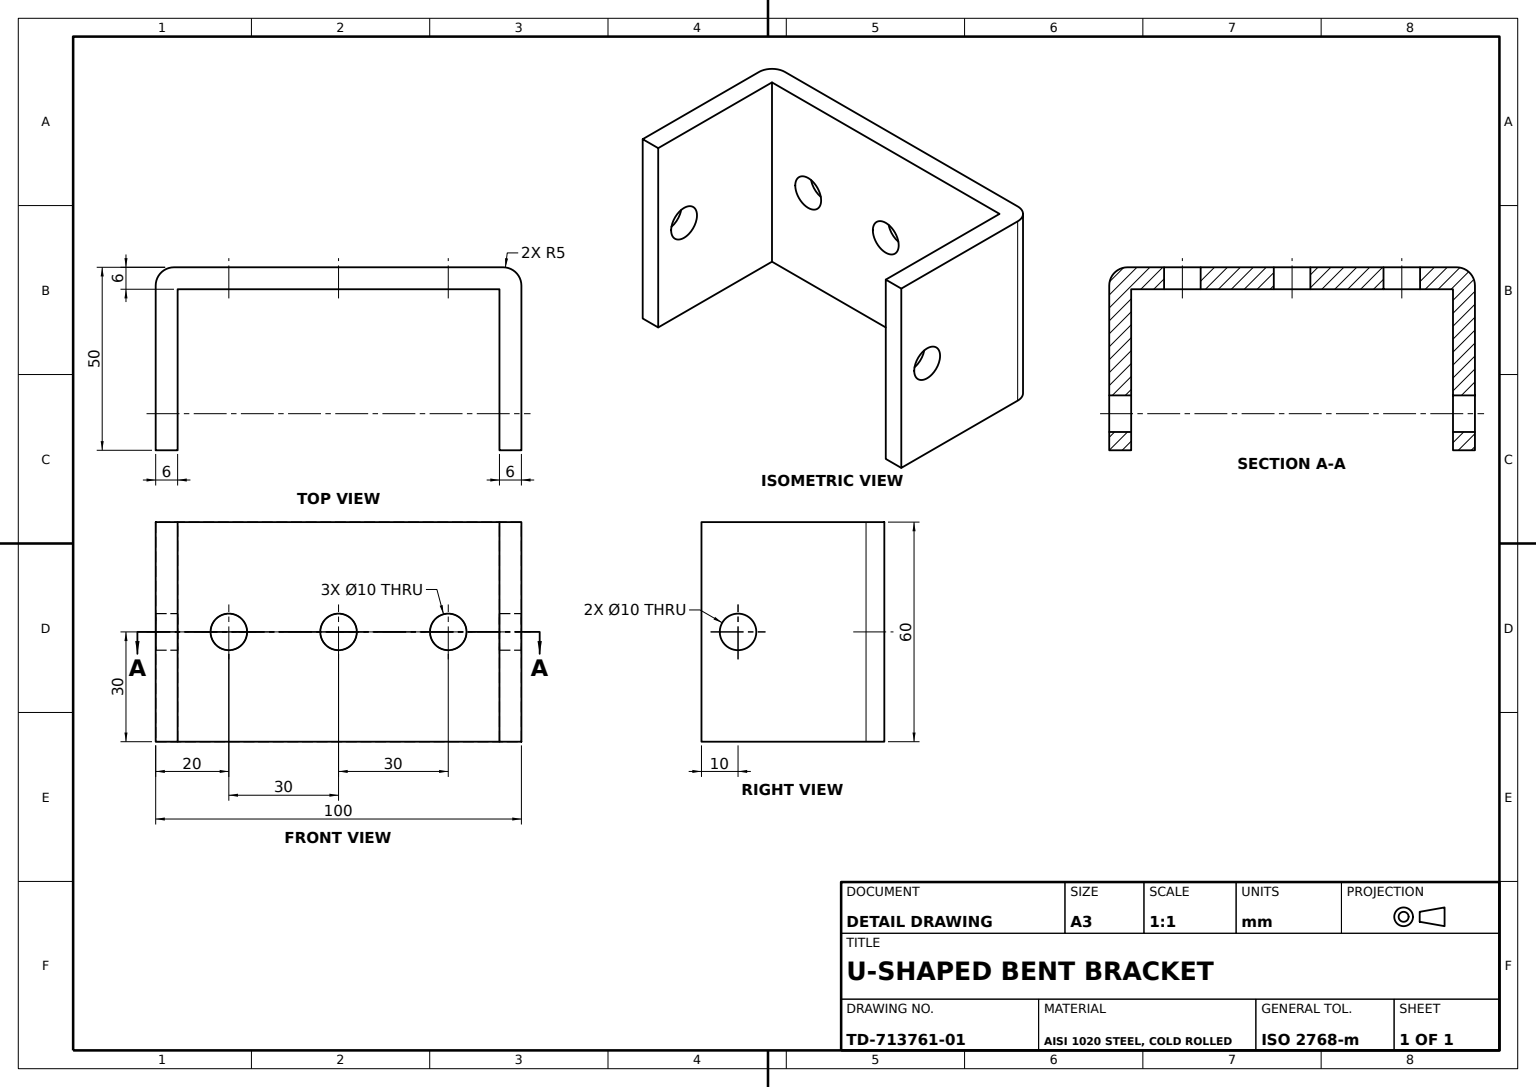
SolidWorks part; units mm, degrees
material "AISI 1020 Steel, Cold Rolled"
ref_plane "Front Plane" through (0, 0, 0) normal (0, 0, 1) x (1, 0, 0)
ref_plane "Top Plane" through (0, 0, 0) normal (0, 1, 0) x (1, 0, 0)
ref_plane "Right Plane" through (0, 0, 0) normal (1, 0, 0) x (0, 0, -1)
sketch "Channel Profile Sketch" plane through (0, 0, 0) normal (0, 1, 0) x (1, 0, 0)
  line L0 (0, 0) -> (0, 50)
  line L1 (0, 50) -> (100, 50)
  line L2 (100, 50) -> (100, 0)
  line L4 (100, 0) -> (94, 0)
  line L5 (94, 0) -> (94, 44)
  line L6 (94, 44) -> (6, 44)
  line L7 (6, 44) -> (6, 0)
  line L8 (6, 0) -> (0, 0)
  dimension "D1" = 50
  dimension "D2" = 100
  dimension "D3" = 6
  dimension "D4" = 6
  dimension "D5" = 6
extrude "Channel Body" add sketch "Channel Profile Sketch" against normal mid plane 60
sketch "Flange Holes Sketch" plane through (0, 0, -50) normal (0, 0, -1) x (-1, 0, 0)
  line L0 (0, 0) -> (-343.6549, 0) construction
  line L1 (-50, -30) -> (-50, 63.2025) construction
  line L2 (-100, -30) -> (0, -30) construction
  circle A0 centre (-50, 0) radius 5
  circle A1 centre (-20, 0) radius 5
  circle A2 centre (-80, 0) radius 5
  dimension "D1" = 60
  dimension "D2" = 10
extrude "Flange Holes" cut sketch "Flange Holes Sketch" against normal mid plane 60
sketch "Back Wall Hole Sketch" plane through (100, 0, 0) normal (1, 0, 0) x (0, 0, -1)
  line L0 (0, -30) -> (0, 30) construction
  line L1 (0, 30) -> (50, 30) construction
  circle A0 centre (10, 0) radius 5
  dimension "D2" = 10
  dimension "D1" = 10
  dimension "D3" = 30
extrude "Back Wall Holes" cut sketch "Back Wall Hole Sketch" against normal up to surface (100 mm away) up to face at (0, 0, -25)
fillet "Corner Fillets R5" radius 5 2 edges at (100, 0, -50) (0, 0, -50)
